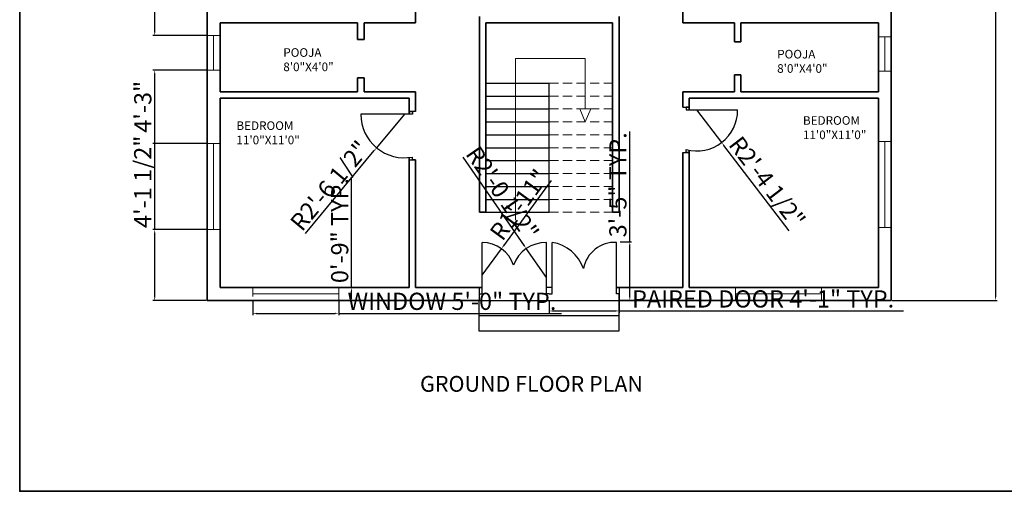
# Model space of a CAD drawing. Units: inches. Extents: x 2142 to 3604, y 1690 to 2981.
# Tile 1 of 9: x 2142 to 2829, y 1690 to 2019. Entities that reach past the tile are written whole.
import ezdxf

# ---------------------------------------------------------------- set-up
doc = ezdxf.new("R2010")
doc.units = ezdxf.units.IN
doc.linetypes.add('DASHED2', pattern=[9.525, 6.35, -3.175])
for name, color, linetype, lineweight in [('A-ANNO-DIMS', 2, 'Continuous', 18), ('A-ANNO-SYMB', 7, 'Continuous', 18), ('A-ANNO-TEXT', 7, 'Continuous', 18), ('A-ANNO-TTLB', 7, 'Continuous', 35), ('A-AREA-IDEN', 7, 'Continuous', 18), ('A-DOOR', 4, 'Continuous', 25), ('A-FLOR-STRS', 7, 'Continuous', 25), ('A-FLOR-STRS-OVHD', 254, 'DASHED2', 18), ('A-GLAZ', 4, 'Continuous', 18), ('A-GLAZ-HIDN', 254, 'DASHED2', 18), ('A-WALL', 7, 'Continuous', 35)]:
    doc.layers.add(name, color=color, linetype=linetype, lineweight=lineweight)
doc.styles.get("Standard").update_dxf_attribs({"font": 'arial.ttf'})
doc.dimstyles.new('ISO-25', dxfattribs={"dimtxt": 12, "dimasz": 2.5, "dimexe": 1.25, "dimexo": 0.625, "dimtad": 1, "dimdec": 0, "dimlunit": 3, "dimtxsty": 'Standard', "dimcen": 2.5, "dimadec": 0, "dimazin": 0, "dimtfac": 1, "dimtdec": 0, "dimtmove": 0, "dimatfit": 3, "dimfxl": 1, "dimarcsym": 0})

# ---------------------------------------------------------------- blocks, each defined once
blk = doc.blocks.new('*D2')
at = {"layer": 'A-ANNO-DIMS', "color": 0, "lineweight": -2, "transparency": 16777216}
for p, q in [((2751.11, 2415.7), (2824.38, 2415.7)), ((2823.13, 2413.2), (2823.13, 1825.7)), ((2751.11, 1823.2), (2824.38, 1823.2))]:
    blk.add_line(p, q, dxfattribs=at)
at = {"layer": 'A-ANNO-DIMS', "color": 0, "transparency": 16777216}
for points in [[(2822.72, 2413.2), (2823.55, 2413.2), (2823.13, 2415.7)], [(2822.72, 1825.7), (2823.55, 1825.7), (2823.13, 1823.2)]]:
    blk.add_solid(points, dxfattribs=at)
at = {"layer": 'Defpoints', "color": 0, "transparency": 16777216}
for p in [(2750.49, 2415.7), (2750.49, 1823.2), (2823.13, 1823.2)]:
    blk.add_point(p, dxfattribs=at)
at = {"layer": 'A-ANNO-DIMS', "color": 0, "transparency": 16777216, "insert": (2816.38, 2119.45), "char_height": 12, "attachment_point": 5, "rotation": 90}
blk.add_mtext("50'", dxfattribs=at)
blk = doc.blocks.new('DOOR-BED-FRONT-R')
for p, q in [((0, 31.64), (4.5, 31.64)), ((4.5, 31.64), (2.25, 31.64)), ((2.25, 31.64), (2.25, 29.64)), ((2.25, 29.64), (38.25, 29.64)), ((2.25, 0), (2.25, 2)), ((0, 0), (4.5, 0)), ((4.5, 0), (2.25, 0))]:
    blk.add_line(p, q)
blk.add_arc((9.64, 29.64), 28.61, 255.03948, 0)
blk = doc.blocks.new('DOOR-BED-FRONT-L')
for p, q in [((36, 31.84), (0, 31.84)), ((38.25, 33.84), (33.75, 33.84)), ((33.75, 33.84), (36, 33.84)), ((36, 33.84), (36, 31.84)), ((33.75, 0), (38.25, 0)), ((36, 0), (36, 2)), ((38.25, 0), (36, 0))]:
    blk.add_line(p, q)
blk.add_arc((30.37, 31.84), 30.37, 180, 280.68489)
blk = doc.blocks.new('DOOR-ENTRY-PAIR-L')
for p, q in [((2, 4.5), (2, 40.5)), ((46.88, 4.5), (46.88, 40.5)), ((0, 9), (0, 0)), ((0, 4.5), (2, 4.5)), ((48.88, 4.5), (46.88, 4.5))]:
    blk.add_line(p, q)
for centre, radius, start, end in [((2, 17.55), 22.95, 17.70587, 90), ((46.88, 15.91), 24.59, 90, 159.47898)]:
    blk.add_arc(centre, radius, start, end)
blk = doc.blocks.new('DOOR-ENTRY-PAIR-R')
for p, q in [((2, 4.5), (2, 40.5)), ((46.89, 4.5), (46.89, 40.5)), ((48.89, 9), (48.89, 0)), ((0, 4.5), (2, 4.5)), ((48.89, 4.5), (46.89, 4.5)), ((48.89, 0), (48.89, 4.5))]:
    blk.add_line(p, q)
for centre, radius, start, end in [((-2.51, 12.76), 28.1, 19.96217, 80.77047), ((46.01, 17.98), 22.54, 87.78446, 168.79388)]:
    blk.add_arc(centre, radius, start, end)
blk = doc.blocks.new('STEP-ENTRY')
blk.add_line((97.55, 10.76), (0, 10.76))
blk.add_lwpolyline([(0, 21.52), (97.55, 21.52), (97.55, 0), (0, 0)], close=True)
blk = doc.blocks.new('WINDOW-60')
for p, q in [((0, 60), (9, 60)), ((9, 60), (4.5, 60)), ((4.5, 60), (4.5, 0)), ((4.5, 0), (0, 0)), ((0, 0), (9, 0))]:
    blk.add_line(p, q)
blk = doc.blocks.new('WINDOW-24')
for p, q in [((0, 24), (9, 24)), ((9, 24), (4.5, 24)), ((4.5, 24), (4.5, 0)), ((4.5, 0), (0, 0)), ((0, 0), (9, 0))]:
    blk.add_line(p, q)
blk = doc.blocks.new('WINDOW-60-ENTRY')
for p, q in [((60, 4.5), (60, 9)), ((60, 9), (60, 0)), ((0, 4.5), (60, 4.5))]:
    blk.add_line(p, q)
blk = doc.blocks.new('STAIR-RETURN-ARROW')
for p, q in [((0, 0), (0, 112.66)), ((0, 112.66), (48.8, 112.66)), ((48.8, 112.66), (48.8, 77.43)), ((52.73, 77.43), (44.99, 77.43)), ((44.99, 77.43), (48.8, 68.43)), ((48.8, 68.43), (52.73, 77.43)), ((48.8, 68.43), (48.8, 68.43))]:
    blk.add_line(p, q)
blk = doc.blocks.new('*D39')
at = {"layer": 'A-ANNO-DIMS', "color": 0, "lineweight": -2, "transparency": 16777216}
for p, q in [((2304.76, 1822.57), (2304.76, 1812.95)), ((2364.76, 1822.57), (2364.76, 1812.95)), ((2307.26, 1814.2), (2362.26, 1814.2)), ((2364.76, 1814.2), (2520.36, 1814.2))]:
    blk.add_line(p, q, dxfattribs=at)
at = {"layer": 'A-ANNO-DIMS', "color": 0, "transparency": 16777216}
for points in [[(2307.26, 1814.61), (2307.26, 1813.78), (2304.76, 1814.2)], [(2362.26, 1814.61), (2362.26, 1813.78), (2364.76, 1814.2)]]:
    blk.add_solid(points, dxfattribs=at)
at = {"layer": 'Defpoints', "color": 0, "transparency": 16777216}
for p in [(2304.76, 1823.2), (2364.76, 1823.2), (2364.76, 1814.2)]:
    blk.add_point(p, dxfattribs=at)
at = {"layer": 'A-ANNO-DIMS', "color": 0, "transparency": 16777216, "insert": (2443.81, 1821.03), "char_height": 12, "attachment_point": 5}
blk.add_mtext('WINDOW 5\'-0" TYP.', dxfattribs=at)
blk = doc.blocks.new('*D40')
at = {"layer": 'A-ANNO-DIMS', "color": 0, "lineweight": -2, "transparency": 16777216}
for p, q in [((2373.76, 1832.2), (2373.76, 1909.09)), ((2365.38, 1832.2), (2375.01, 1832.2)), ((2373.76, 1825.7), (2373.76, 1829.7)), ((2365.38, 1823.2), (2375.01, 1823.2))]:
    blk.add_line(p, q, dxfattribs=at)
at = {"layer": 'A-ANNO-DIMS', "color": 0, "transparency": 16777216}
for points in [[(2373.34, 1829.7), (2374.17, 1829.7), (2373.76, 1832.2)], [(2373.34, 1825.7), (2374.17, 1825.7), (2373.76, 1823.2)]]:
    blk.add_solid(points, dxfattribs=at)
at = {"layer": 'Defpoints', "color": 0, "transparency": 16777216}
for p in [(2364.76, 1832.2), (2373.76, 1832.2), (2364.76, 1823.2)]:
    blk.add_point(p, dxfattribs=at)
at = {"layer": 'A-ANNO-DIMS', "color": 0, "transparency": 16777216, "insert": (2367.01, 1871.89), "char_height": 12, "attachment_point": 5, "rotation": 90}
blk.add_mtext('0\'-9" TYP.', dxfattribs=at)
blk = doc.blocks.new('*D65')
at = {"layer": 'A-ANNO-DIMS', "color": 0, "lineweight": -2, "transparency": 16777216}
for p, q in [((2511.74, 1822.57), (2511.74, 1814.61)), ((2560.62, 1822.57), (2560.62, 1814.61)), ((2514.24, 1815.86), (2558.12, 1815.86)), ((2560.62, 1815.86), (2758.94, 1815.86))]:
    blk.add_line(p, q, dxfattribs=at)
at = {"layer": 'A-ANNO-DIMS', "color": 0, "transparency": 16777216}
for points in [[(2514.24, 1816.28), (2514.24, 1815.45), (2511.74, 1815.86)], [(2558.12, 1816.28), (2558.12, 1815.45), (2560.62, 1815.86)]]:
    blk.add_solid(points, dxfattribs=at)
at = {"layer": 'Defpoints', "color": 0, "transparency": 16777216}
for p in [(2511.74, 1823.2), (2560.62, 1823.2), (2560.62, 1815.86)]:
    blk.add_point(p, dxfattribs=at)
at = {"layer": 'A-ANNO-DIMS', "color": 0, "transparency": 16777216, "insert": (2661.03, 1822.7), "char_height": 12, "attachment_point": 5}
blk.add_mtext('PAIRED DOOR 4\'-1" TYP.', dxfattribs=at)
blk = doc.blocks.new('*D66')
at = {"layer": 'A-ANNO-DIMS', "color": 0, "lineweight": -2, "transparency": 16777216}
for p, q in [((2567.96, 1864.13), (2567.96, 1941.01)), ((2561.25, 1864.13), (2569.21, 1864.13)), ((2567.96, 1825.7), (2567.96, 1861.63)), ((2561.25, 1823.2), (2569.21, 1823.2))]:
    blk.add_line(p, q, dxfattribs=at)
at = {"layer": 'A-ANNO-DIMS', "color": 0, "transparency": 16777216}
for points in [[(2567.54, 1861.63), (2568.37, 1861.63), (2567.96, 1864.13)], [(2567.54, 1825.7), (2568.37, 1825.7), (2567.96, 1823.2)]]:
    blk.add_solid(points, dxfattribs=at)
at = {"layer": 'Defpoints', "color": 0, "transparency": 16777216}
for p in [(2560.62, 1864.13), (2567.96, 1864.13), (2560.62, 1823.2)]:
    blk.add_point(p, dxfattribs=at)
at = {"layer": 'A-ANNO-DIMS', "color": 0, "transparency": 16777216, "insert": (2561.2, 1903.82), "char_height": 12, "attachment_point": 5, "rotation": 90}
blk.add_mtext('3\'-5" TYP.', dxfattribs=at)
blk = doc.blocks.new('*D98')
at = {"layer": 'A-ANNO-DIMS', "color": 0, "lineweight": -2, "transparency": 16777216}
for p, q in [((2236.34, 1872.64), (2236.34, 1936.73)), ((2272.36, 1872.64), (2235.09, 1872.64)), ((2236.34, 1825.7), (2236.34, 1870.14)), ((2272.36, 1823.2), (2235.09, 1823.2))]:
    blk.add_line(p, q, dxfattribs=at)
at = {"layer": 'A-ANNO-DIMS', "color": 0, "transparency": 16777216}
for points in [[(2235.92, 1870.14), (2236.75, 1870.14), (2236.34, 1872.64)], [(2235.92, 1825.7), (2236.75, 1825.7), (2236.34, 1823.2)]]:
    blk.add_solid(points, dxfattribs=at)
at = {"layer": 'Defpoints', "color": 0, "transparency": 16777216}
for p in [(2236.34, 1872.64), (2272.99, 1872.64), (2272.99, 1823.2)]:
    blk.add_point(p, dxfattribs=at)
at = {"layer": 'A-ANNO-DIMS', "color": 0, "transparency": 16777216, "insert": (2229.51, 1905.94), "char_height": 12, "attachment_point": 5, "rotation": 90}
blk.add_mtext('4\'-1 1/2"', dxfattribs=at)
blk = doc.blocks.new('*D99')
at = {"layer": 'A-ANNO-DIMS', "color": 0, "lineweight": -2, "transparency": 16777216}
for p, q in [((2272.36, 1983.83), (2235.09, 1983.83)), ((2236.34, 1935.14), (2236.34, 1981.33)), ((2272.36, 1932.64), (2235.09, 1932.64))]:
    blk.add_line(p, q, dxfattribs=at)
at = {"layer": 'A-ANNO-DIMS', "color": 0, "transparency": 16777216}
for points in [[(2235.92, 1981.33), (2236.75, 1981.33), (2236.34, 1983.83)], [(2235.92, 1935.14), (2236.75, 1935.14), (2236.34, 1932.64)]]:
    blk.add_solid(points, dxfattribs=at)
at = {"layer": 'Defpoints', "color": 0, "transparency": 16777216}
for p in [(2236.34, 1983.83), (2272.99, 1983.83), (2272.99, 1932.64)]:
    blk.add_point(p, dxfattribs=at)
at = {"layer": 'A-ANNO-DIMS', "color": 0, "transparency": 16777216, "insert": (2229.58, 1958.23), "char_height": 12, "attachment_point": 5, "rotation": 90}
blk.add_mtext('4\'-3"', dxfattribs=at)
blk = doc.blocks.new('*D100')
at = {"layer": 'A-ANNO-DIMS', "color": 0, "lineweight": -2, "transparency": 16777216}
for p, q in [((2236.34, 2059.45), (2236.34, 2123.54)), ((2272.36, 2059.45), (2235.09, 2059.45)), ((2236.34, 2010.33), (2236.34, 2056.95)), ((2272.36, 2007.83), (2235.09, 2007.83))]:
    blk.add_line(p, q, dxfattribs=at)
at = {"layer": 'A-ANNO-DIMS', "color": 0, "transparency": 16777216}
for points in [[(2235.92, 2056.95), (2236.75, 2056.95), (2236.34, 2059.45)], [(2235.92, 2010.33), (2236.75, 2010.33), (2236.34, 2007.83)]]:
    blk.add_solid(points, dxfattribs=at)
at = {"layer": 'Defpoints', "color": 0, "transparency": 16777216}
for p in [(2236.34, 2059.45), (2272.99, 2059.45), (2272.99, 2007.83)]:
    blk.add_point(p, dxfattribs=at)
at = {"layer": 'A-ANNO-DIMS', "color": 0, "transparency": 16777216, "insert": (2229.5, 2092.74), "char_height": 12, "attachment_point": 5, "rotation": 90}
blk.add_mtext('4\'-3 1/2"', dxfattribs=at)
blk = doc.blocks.new('*D125')
at = {"layer": 'A-ANNO-DIMS', "color": 0, "lineweight": -2, "transparency": 16777216}
for p, q in [((2410.61, 1953.05), (2391.22, 1929.67)), ((2341.7, 1869.93), (2389.63, 1927.74))]:
    blk.add_line(p, q, dxfattribs=at)
at = {"layer": 'A-ANNO-DIMS', "color": 0, "transparency": 16777216}
blk.add_solid([(2389.31, 1928.01), (2389.95, 1927.48), (2391.22, 1929.67)], dxfattribs=at)
at = {"layer": 'Defpoints', "color": 0, "transparency": 16777216}
for p in [(2410.61, 1953.05), (2391.22, 1929.67)]:
    blk.add_point(p, dxfattribs=at)
at = {"layer": 'A-ANNO-DIMS', "color": 0, "transparency": 16777216, "insert": (2359.61, 1902.23), "char_height": 12, "attachment_point": 5, "rotation": 50.34156}
blk.add_mtext('R2\'-6 1/2"', dxfattribs=at)
blk = doc.blocks.new('*D128')
at = {"layer": 'A-ANNO-DIMS', "color": 0, "lineweight": -2, "transparency": 16777216}
for p, q in [((2614.62, 1956.02), (2632.05, 1933.32)), ((2679.31, 1871.78), (2633.57, 1931.34))]:
    blk.add_line(p, q, dxfattribs=at)
at = {"layer": 'A-ANNO-DIMS', "color": 0, "transparency": 16777216}
blk.add_solid([(2633.9, 1931.59), (2633.24, 1931.09), (2632.05, 1933.32)], dxfattribs=at)
at = {"layer": 'Defpoints', "color": 0, "transparency": 16777216}
for p in [(2614.62, 1956.02), (2632.05, 1933.32)]:
    blk.add_point(p, dxfattribs=at)
at = {"layer": 'A-ANNO-DIMS', "color": 0, "transparency": 16777216, "insert": (2662.62, 1904.73), "char_height": 12, "attachment_point": 5, "rotation": 307.52042}
blk.add_mtext('R2\'-4 1/2"', dxfattribs=at)
blk = doc.blocks.new('*D130')
at = {"layer": 'A-ANNO-DIMS', "color": 0, "lineweight": -2, "transparency": 16777216}
for p, q in [((2451.51, 1923.08), (2494.3, 1861.37)), ((2509.74, 1839.11), (2495.73, 1859.31))]:
    blk.add_line(p, q, dxfattribs=at)
at = {"layer": 'A-ANNO-DIMS', "color": 0, "transparency": 16777216}
blk.add_solid([(2494.64, 1861.61), (2493.96, 1861.13), (2495.73, 1859.31)], dxfattribs=at)
at = {"layer": 'Defpoints', "color": 0, "transparency": 16777216}
for p in [(2495.73, 1859.31), (2509.74, 1839.11)]:
    blk.add_point(p, dxfattribs=at)
at = {"layer": 'A-ANNO-DIMS', "color": 0, "transparency": 16777216, "insert": (2477.81, 1897.14), "char_height": 12, "attachment_point": 5, "rotation": 304.73982}
blk.add_mtext('R2\'-0 1/2"', dxfattribs=at)
blk = doc.blocks.new('*D132')
at = {"layer": 'A-ANNO-DIMS', "color": 0, "lineweight": -2, "transparency": 16777216}
for p, q in [((2513.16, 1906.89), (2479.86, 1861.3)), ((2464.85, 1840.75), (2478.39, 1859.28))]:
    blk.add_line(p, q, dxfattribs=at)
at = {"layer": 'A-ANNO-DIMS', "color": 0, "transparency": 16777216}
blk.add_solid([(2479.53, 1861.54), (2480.2, 1861.05), (2478.39, 1859.28)], dxfattribs=at)
at = {"layer": 'Defpoints', "color": 0, "transparency": 16777216}
for p in [(2478.39, 1859.28), (2464.85, 1840.75)]:
    blk.add_point(p, dxfattribs=at)
at = {"layer": 'A-ANNO-DIMS', "color": 0, "transparency": 16777216, "insert": (2491.88, 1889.02), "char_height": 12, "attachment_point": 5, "rotation": 53.85259}
blk.add_mtext('R1\'-11"', dxfattribs=at)

msp = doc.modelspace()

# ---------------------------------------------------------------- linework, layer by layer
at = {"layer": 'A-ANNO-TTLB'}
msp.add_lwpolyline([(2142.1, 2981.01), (3604.42, 2981.01), (3604.42, 1690.13), (2142.1, 1690.13)], close=True, dxfattribs=at)
at = {"layer": 'A-DOOR'}
msp.add_line((2513.74, 1832.2), (2509.74, 1832.2), dxfattribs=at)
at = {"layer": 'A-FLOR-STRS'}
for p, q in [((2467.49, 1974.7), (2511.74, 1974.7)), ((2511.74, 1884.7), (2511.74, 1974.7)), ((2467.49, 1965.7), (2511.74, 1965.7)), ((2467.49, 1956.7), (2511.74, 1956.7)), ((2467.49, 1947.7), (2511.74, 1947.7)), ((2467.49, 1938.7), (2511.74, 1938.7)), ((2467.49, 1929.7), (2511.74, 1929.7)), ((2467.49, 1920.7), (2511.74, 1920.7)), ((2467.49, 1911.7), (2511.74, 1911.7)), ((2467.49, 1902.7), (2511.74, 1902.7)), ((2467.49, 1893.7), (2511.74, 1893.7)), ((2467.49, 1884.7), (2511.74, 1884.7))]:
    msp.add_line(p, q, dxfattribs=at)
at = {"layer": 'A-FLOR-STRS-OVHD'}
for p, q in [((2511.74, 1974.7), (2555.99, 1974.7)), ((2511.74, 1965.7), (2555.99, 1965.7)), ((2511.74, 1956.7), (2555.99, 1956.7)), ((2511.74, 1947.7), (2555.99, 1947.7)), ((2511.74, 1938.7), (2555.99, 1938.7)), ((2511.74, 1929.7), (2555.99, 1929.7)), ((2511.74, 1920.7), (2555.99, 1920.7)), ((2511.74, 1911.7), (2555.99, 1911.7)), ((2511.74, 1902.7), (2555.99, 1902.7)), ((2511.74, 1893.7), (2555.99, 1893.7)), ((2511.74, 1884.7), (2555.99, 1884.7))]:
    msp.add_line(p, q, dxfattribs=at)
at = {"layer": 'A-GLAZ-HIDN'}
msp.add_line((2304.76, 1832.2), (2304.76, 1823.2), dxfattribs=at)
at = {"layer": 'A-WALL'}
for p, q in [((2272.99, 2415.7), (2272.99, 1823.2)), ((2750.49, 2415.7), (2750.49, 1823.2)), ((2418.49, 2157.29), (2418.49, 2016.7)), ((2604.99, 2157.7), (2604.99, 2016.7)), ((2462.99, 1884.7), (2462.99, 2021.2)), ((2560.49, 1884.7), (2560.49, 2021.2)), ((2281.99, 2016.7), (2377.99, 2016.7)), ((2281.99, 2016.7), (2281.99, 1968.7)), ((2377.99, 2005.04), (2377.99, 2016.7)), ((2382.49, 2005.04), (2382.49, 2016.7)), ((2382.49, 2016.7), (2418.49, 2016.7)), ((2509.49, 2016.7), (2467.49, 2016.7)), ((2467.49, 2016.7), (2467.49, 1884.7)), ((2467.49, 2016.7), (2555.99, 2016.7)), ((2513.99, 2016.7), (2555.99, 2016.7)), ((2555.99, 2016.7), (2555.99, 1884.7)), ((2640.99, 2016.7), (2604.99, 2016.7)), ((2640.99, 2016.7), (2640.99, 2003.42)), ((2741.49, 2016.7), (2645.49, 2016.7)), ((2645.49, 2003.42), (2645.49, 2016.7)), ((2741.49, 2016.7), (2741.49, 1968.7)), ((2377.99, 2005.04), (2382.49, 2005.04)), ((2640.99, 2003.42), (2645.49, 2003.42)), ((2640.99, 1980.46), (2645.49, 1980.46)), ((2640.99, 1980.46), (2640.99, 1968.7)), ((2645.49, 1968.7), (2645.49, 1980.46)), ((2377.99, 1968.7), (2377.99, 1978.38)), ((2377.99, 1978.38), (2382.49, 1978.38)), ((2382.49, 1968.7), (2382.49, 1978.38)), ((2281.99, 1968.7), (2377.99, 1968.7)), ((2382.49, 1968.7), (2418.49, 1968.7)), ((2418.49, 1968.7), (2418.49, 1955.05)), ((2604.99, 1968.7), (2604.99, 1958.02)), ((2640.99, 1968.7), (2604.99, 1968.7)), ((2741.49, 1968.7), (2645.49, 1968.7)), ((2741.49, 1968.7), (2645.49, 1968.7)), ((2281.99, 1964.2), (2413.99, 1964.2)), ((2281.99, 1964.2), (2413.99, 1964.2)), ((2281.99, 1964.2), (2281.99, 1832.2)), ((2377.99, 1964.2), (2382.49, 1964.2)), ((2413.99, 1964.2), (2413.99, 1953.05)), ((2741.49, 1964.2), (2609.49, 1964.2)), ((2609.49, 1964.2), (2609.49, 1956.02)), ((2741.49, 1964.2), (2741.49, 1832.2)), ((2604.99, 1926.37), (2604.99, 1832.2)), ((2609.49, 1927.87), (2609.49, 1832.2)), ((2413.99, 1922.87), (2413.99, 1832.2)), ((2418.49, 1921.2), (2418.49, 1832.2)), ((2467.49, 1884.7), (2462.99, 1884.7)), ((2555.99, 1884.7), (2560.49, 1884.7)), ((2413.99, 1832.2), (2281.99, 1832.2)), ((2464.85, 1832.2), (2418.49, 1832.2)), ((2604.99, 1832.2), (2558.62, 1832.2)), ((2741.49, 1832.2), (2609.49, 1832.2)), ((2462.85, 1823.2), (2272.99, 1823.2)), ((2750.49, 1823.2), (2560.62, 1823.2))]:
    msp.add_line(p, q, dxfattribs=at)

# ---------------------------------------------------------------- block references
at = {"layer": 'A-ANNO-SYMB'}
msp.add_blockref('STAIR-RETURN-ARROW', (2488.1, 1879.26), dxfattribs=at)
at = {"layer": 'A-DOOR'}
for name, p in [('DOOR-BED-FRONT-L', (2380.24, 1921.2)), ('DOOR-BED-FRONT-R', (2604.99, 1926.37)), ('DOOR-ENTRY-PAIR-L', (2462.85, 1823.2)), ('DOOR-ENTRY-PAIR-R', (2511.74, 1823.2))]:
    msp.add_blockref(name, p, dxfattribs=at)
at = {"layer": 'A-FLOR-STRS'}
msp.add_blockref('STEP-ENTRY', (2462.85, 1801.68), dxfattribs=at)
at = {"layer": 'A-GLAZ'}
for name, p in [('WINDOW-24', (2272.99, 1983.83)), ('WINDOW-24', (2741.49, 1983.01)), ('WINDOW-60', (2272.99, 1872.64)), ('WINDOW-60', (2741.49, 1874.08)), ('WINDOW-60-ENTRY', (2304.76, 1823.2))]:
    msp.add_blockref(name, p, dxfattribs=at)
at = {"layer": 'A-GLAZ', "extrusion": (0, 0, -1), "zscale": -1, "rotation": 270}
msp.add_blockref('WINDOW-60', (-2701.76, 1832.2), dxfattribs=at)

# ---------------------------------------------------------------- texts
at = {"layer": 'A-ANNO-TEXT', "insert": (2421.57, 1770.52), "char_height": 11, "attachment_point": 1}
msp.add_mtext_dynamic_manual_height_columns('GROUND FLOOR PLAN', width=393.8468, gutter_width=12.5, heights=[0], dxfattribs=at)
at = {"layer": 'A-AREA-IDEN', "char_height": 6, "attachment_point": 1}
for s, width, insert in [('POOJA\\P8\'0"X4\'0"', 88.9099, (2326.08, 1999.07)), ('POOJA\\P8\'0"X4\'0"', 88.9099, (2670.83, 1997.93)), ('BEDROOM\\P11\'0"X11\'0"', 99.4346, (2293.36, 1948.08)), ('BEDROOM\\P11\'0"X11\'0"', 99.4346, (2688.82, 1951.69))]:
    msp.add_mtext_dynamic_manual_height_columns(s, width=width, gutter_width=12.5, heights=[0], dxfattribs=dict(at, insert=insert))

# ---------------------------------------------------------------- dimensions: what is measured, and where the dimension line sits
at = {"layer": 'A-ANNO-DIMS'}
for base, p1, p2, text, override, picture, middle in [((2823.13, 1823.2), (2750.49, 2415.7), (2750.49, 1823.2), "50'", {"dimclrd": 0, "dimclre": 0, "dimclrt": 0}, '*D2', (2816.38, 2119.45)), ((2567.96, 1864.13), (2560.62, 1823.2), (2560.62, 1864.13), '<> TYP.', {"dimdec": 1, "dimlfac": 1, "dimrnd": 0, "dimzin": 1, "dimdsep": 46, "dimlunit": 4, "dimfrac": 2}, '*D66', (2561.2, 1903.82)), ((2373.76, 1832.2), (2364.76, 1823.2), (2364.76, 1832.2), '<> TYP.', {"dimdec": 1, "dimlfac": 1, "dimrnd": 0, "dimzin": 1, "dimdsep": 46, "dimlunit": 4, "dimfrac": 2}, '*D40', (2367.01, 1871.89))]:
    dim = msp.add_linear_dim(base=base, p1=p1, p2=p2, angle=90, text=text, dimstyle='ISO-25', override=override, dxfattribs=at)
    dim.commit()
    dim.dimension.update_dxf_attribs({"geometry": picture, "text_midpoint": middle})
for base, p1, p2, picture, middle in [((2236.34, 2059.45), (2272.99, 2007.83), (2272.99, 2059.45), '*D100', (2229.5, 2092.74)), ((2236.34, 1983.83), (2272.99, 1932.64), (2272.99, 1983.83), '*D99', (2229.58, 1958.23)), ((2236.34, 1872.64), (2272.99, 1823.2), (2272.99, 1872.64), '*D98', (2229.51, 1905.94))]:
    dim = msp.add_linear_dim(base=base, p1=p1, p2=p2, angle=90, dimstyle='ISO-25', override={"dimdec": 1, "dimlfac": 1, "dimrnd": 0, "dimzin": 1, "dimdsep": 46, "dimlunit": 4, "dimfrac": 2}, dxfattribs=at)
    dim.commit()
    dim.dimension.update_dxf_attribs({"geometry": picture, "text_midpoint": middle})
for center, mpoint, picture, middle in [((2410.61, 1953.05), (2391.22, 1929.67), '*D125', (2359.61, 1902.23)), ((2614.62, 1956.02), (2632.05, 1933.32), '*D128', (2662.62, 1904.73)), ((2509.74, 1839.11), (2495.73, 1859.31), '*D130', (2477.81, 1897.14)), ((2464.85, 1840.75), (2478.39, 1859.28), '*D132', (2491.88, 1889.02))]:
    dim = msp.add_radius_dim(center=center, mpoint=mpoint, dimstyle='ISO-25', override={"dimdec": 1, "dimlfac": 1, "dimrnd": 0, "dimzin": 1, "dimdsep": 46, "dimlunit": 4, "dimfrac": 2}, dxfattribs=at)
    dim.commit()
    dim.dimension.update_dxf_attribs({"geometry": picture, "text_midpoint": middle})
for base, p1, p2, text, picture, middle in [((2560.62, 1815.86), (2511.74, 1823.2), (2560.62, 1823.2), 'PAIRED DOOR <> TYP.', '*D65', (2661.03, 1822.7)), ((2364.76, 1814.2), (2304.76, 1823.2), (2364.76, 1823.2), 'WINDOW <> TYP.', '*D39', (2443.81, 1821.03))]:
    dim = msp.add_linear_dim(base=base, p1=p1, p2=p2, text=text, dimstyle='ISO-25', override={"dimdec": 1, "dimlfac": 1, "dimrnd": 0, "dimzin": 1, "dimdsep": 46, "dimlunit": 4, "dimfrac": 2}, dxfattribs=at)
    dim.commit()
    dim.dimension.update_dxf_attribs({"geometry": picture, "text_midpoint": middle})

doc.saveas('drawing.dxf')
